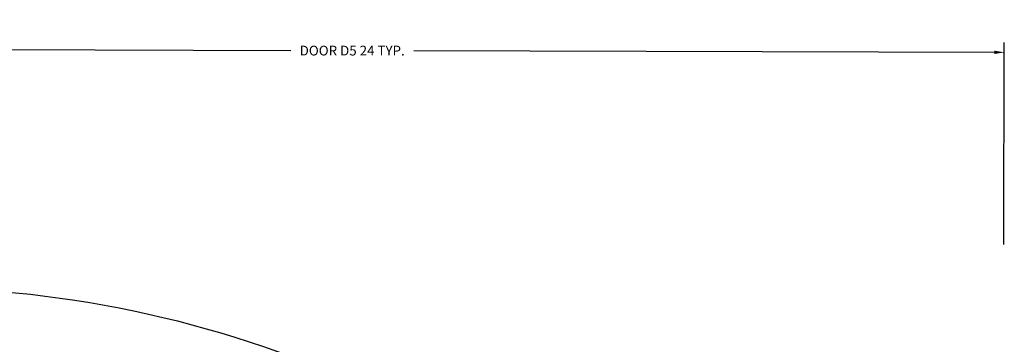
# Model space of a CAD drawing. Units: inches. Extents: x 1901 to 2863, y 888 to 2433.
# Tile 83 of 91: x 2663 to 2681, y 2037 to 2043. Entities that reach past the tile are written whole.
import ezdxf

# ---------------------------------------------------------------- set-up
doc = ezdxf.new("R2010")
doc.units = ezdxf.units.IN
doc.layers.add('A-ANNO-DIMS', color=2, linetype='Continuous', lineweight=18)
doc.layers.add('A-DOOR', color=4, linetype='Continuous', lineweight=25)
doc.styles.get("Standard").update_dxf_attribs({"font": 'arial.ttf'})
doc.dimstyles.get("Standard").update_dxf_attribs({"dimtxt": 0.18, "dimasz": 0.18, "dimexe": 0.18, "dimexo": 0.0625, "dimgap": 0.09, "dimtad": 0, "dimtih": 1, "dimtoh": 1, "dimdec": 4, "dimzin": 0, "dimdsep": 46, "dimtxsty": 'Standard', "dimcen": 0.09, "dimadec": 0, "dimazin": 0, "dimtfac": 1, "dimtdec": 4, "dimtofl": 0, "dimtmove": 0, "dimatfit": 3, "dimfxl": 1, "dimtolj": 1, "dimtzin": 0, "dimarcsym": 0})

# ---------------------------------------------------------------- blocks, each defined once
blk = doc.blocks.new('DOOR-20B')
blk.add_line((0.002, -0.016), (0.002, 23.984))
blk.add_arc((0.002, 3.902), 20.082, 348.7487, 90)
blk = doc.blocks.new('*D39')
at = {"layer": 'A-ANNO-DIMS', "color": 0, "lineweight": -2, "transparency": 16777216}
for p, q in [((2657.208, 2038.63), (2657.218, 2042.347)), ((2681.208, 2038.564), (2681.218, 2042.282)), ((2657.397, 2042.167), (2668.086, 2042.138)), ((2681.037, 2042.102), (2670.349, 2042.131))]:
    blk.add_line(p, q, dxfattribs=at)
at = {"layer": 'A-ANNO-DIMS', "color": 0, "transparency": 16777216}
for points in [[(2657.397, 2042.197), (2657.397, 2042.137), (2657.217, 2042.167)], [(2681.037, 2042.132), (2681.037, 2042.072), (2681.217, 2042.102)]]:
    blk.add_solid(points, dxfattribs=at)
at = {"layer": 'Defpoints', "color": 0, "transparency": 16777216}
for p in [(2681.217, 2042.102), (2657.208, 2038.567), (2681.207, 2038.502)]:
    blk.add_point(p, dxfattribs=at)
at = {"layer": 'A-ANNO-DIMS', "color": 0, "transparency": 16777216, "insert": (2669.217, 2042.134), "char_height": 0.18, "attachment_point": 5}
blk.add_mtext('\\A1;DOOR D5 24 TYP.', dxfattribs=at)

msp = doc.modelspace()

# ---------------------------------------------------------------- block references
at = {"layer": 'A-DOOR', "extrusion": (0, 0, -1), "zscale": -1, "rotation": 90.1553947244059}
msp.add_blockref('DOOR-20B', (-2657.167, 2017.696), dxfattribs=at)

# ---------------------------------------------------------------- dimensions: what is measured, and where the dimension line sits
at = {"layer": 'A-ANNO-DIMS'}
dim = msp.add_linear_dim(base=(2681.217, 2042.102), p1=(2657.208, 2038.567), p2=(2681.207, 2038.502), angle=359.8446, text='DOOR D5 <> TYP.', dimstyle='Standard', override={"dimdec": 0, "dimlfac": 1, "dimrnd": 0, "dimzin": 0, "dimdsep": 46, "dimlunit": 2}, dxfattribs=at)
dim.commit()
dim.dimension.update_dxf_attribs({"geometry": '*D39', "text_midpoint": (2669.217, 2042.134)})

doc.saveas('drawing.dxf')
